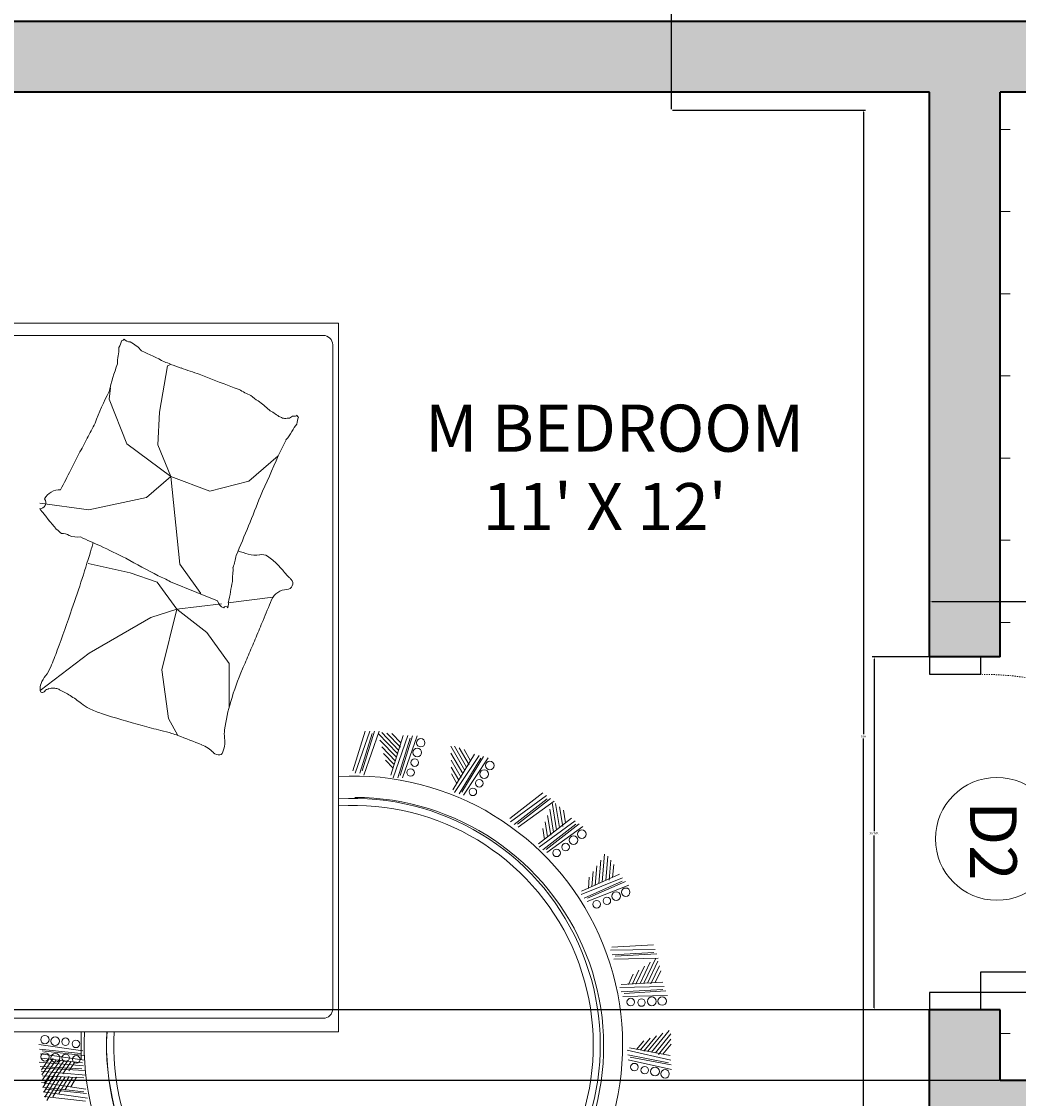
# Model space of a CAD drawing. Units: inches. Extents: x 2701 to 6846, y 811 to 2447.
# Tile 11 of 20: x 2841 to 2926, y 1371 to 1462. Entities that reach past the tile are written whole.
import ezdxf

# ---------------------------------------------------------------- set-up
doc = ezdxf.new("R2010")
doc.units = ezdxf.units.IN
doc.linetypes.add('HIDDEN4', pattern=[0.09375, 0.0625, -0.03125])
for name, color, linetype, lineweight in [('A-ANNO-DIMS', 2, 'Continuous', 18), ('A-ANNO-IDEN', 7, 'Continuous', 13), ('A-AREA-IDEN', 7, 'Continuous', 18), ('A-DOOR', 4, 'Continuous', 25), ('A-DOOR-SWNG', 4, 'HIDDEN4', 13), ('A-FLOR-PATT', 252, 'Continuous', 13), ('A-FURN', 8, 'Continuous', 13), ('A-WALL', 7, 'Continuous', 35)]:
    doc.layers.add(name, color=color, linetype=linetype, lineweight=lineweight)
doc.layers.add('A-WALL-PATT', color=18, linetype='Continuous', lineweight=13, true_color=0x000000)
doc.styles.add('DIM_FONT', font='SIMPLEX.shx', dxfattribs={"width": 0.8})
doc.styles.get("Standard").update_dxf_attribs({"font": 'arial.ttf'})
doc.dimstyles.get("Standard").update_dxf_attribs({"dimtxt": 0.18, "dimasz": 0.18, "dimexe": 0.18, "dimexo": 0.0625, "dimgap": 0.09, "dimtad": 0, "dimtih": 1, "dimtoh": 1, "dimdec": 4, "dimzin": 0, "dimdsep": 46, "dimtxsty": 'Standard', "dimcen": 0.09, "dimadec": 0, "dimazin": 0, "dimtfac": 1, "dimtdec": 4, "dimtofl": 0, "dimtmove": 0, "dimatfit": 3, "dimfxl": 1, "dimtolj": 1, "dimtzin": 0, "dimarcsym": 0})

# ---------------------------------------------------------------- blocks, each defined once
blk = doc.blocks.new('A$C187B6359')
for p, q in [((0.6999, 2.7053), (0.6999, 0.7053)), ((2.1999, 0.7053), (2.1999, 2.7053)), ((2.1741, 2.1968), (2.1741, 0.7375)), ((0.7284, 0.7375), (0.7284, 1.7894)), ((0.5629, 1.3285), (0.5533, 1.2408)), ((0.6047, 1.292), (0.5545, 1.3229)), ((0.5727, 1.3302), (0.5591, 1.2368)), ((0.6051, 1.3), (0.5613, 1.327)), ((0.5785, 1.3262), (0.5689, 1.2385)), ((0.6077, 1.3067), (0.5719, 1.3288)), ((0.5825, 1.332), (0.5729, 1.2443)), ((0.5923, 1.3337), (0.5787, 1.2403)), ((0.6059, 1.3161), (0.5826, 1.3304)), ((0.6394, 1.2947), (0.5911, 1.3283)), ((0.6403, 1.3027), (0.5981, 1.332)), ((0.6068, 1.3321), (0.6021, 1.244)), ((0.6165, 1.3344), (0.6081, 1.2403)), ((0.6432, 1.3092), (0.6087, 1.3332)), ((0.6225, 1.3307), (0.6178, 1.2426)), ((0.642, 1.3186), (0.6195, 1.3342)), ((0.6262, 1.3367), (0.6215, 1.2486)), ((0.6358, 1.339), (0.6275, 1.2449)), ((0.6437, 1.3345), (0.6342, 1.2469)), ((0.6535, 1.3363), (0.6399, 1.2428)), ((0.6593, 1.3323), (0.6497, 1.2446)), ((0.6633, 1.3381), (0.6538, 1.2504)), ((0.6731, 1.3398), (0.6595, 1.2463)), ((1.4224, 1.3369), (1.5015, 1.233)), ((1.8189, 1.3371), (1.8052, 1.2339)), ((0.6042, 1.284), (0.5618, 1.3102)), ((0.6385, 1.2867), (0.5976, 1.3152)), ((0.6387, 1.278), (0.6041, 1.3021)), ((0.6049, 1.2753), (0.569, 1.2975)), ((0.6034, 1.268), (0.5762, 1.2848)), ((0.6368, 1.2708), (0.6105, 1.289)), ((0.6035, 1.2597), (0.5834, 1.2721)), ((0.6364, 1.2624), (0.617, 1.2759)), ((0.6999, 1.25), (0.641, 1.25)), ((1.5015, 1.233), (1.5767, 1.1026)), ((1.6715, 1.1461), (1.6913, 1.235)), ((1.8052, 1.2339), (1.831, 1.1119)), ((1.9445, 1.1532), (2.0391, 1.191)), ((2.0391, 1.191), (2.0632, 1.1875)), ((1.6518, 1.0888), (1.6715, 1.1461)), ((1.8757, 1.0603), (1.9445, 1.1532)), ((1.5767, 1.1026), (1.5944, 1.0473)), ((1.831, 1.1119), (1.8757, 1.0603)), ((1.466, 1.0789), (1.3632, 1.0651)), ((1.5944, 1.0473), (1.466, 1.0789)), ((1.5944, 1.0473), (1.6518, 1.0888)), ((1.8757, 1.0603), (1.9428, 1.0878)), ((1.9428, 1.0878), (2.0116, 1.0844)), ((2.0116, 1.0844), (2.1096, 1.0672)), ((1.3632, 1.0651), (1.3272, 1.045)), ((1.6527, 1.0611), (1.6296, 1.0048)), ((1.8757, 1.0603), (1.6899, 1.0414)), ((1.8447, 0.9778), (1.8757, 1.0603)), ((2.1096, 1.0672), (2.1129, 1.0608)), ((1.545, 0.9841), (1.5944, 1.0473)), ((1.5944, 1.0473), (1.6062, 0.9532)), ((1.6899, 1.0414), (1.64, 1.0053)), ((1.6296, 1.0048), (1.6119, 0.9614)), ((1.64, 1.0053), (1.628, 0.9967)), ((1.4798, 0.9367), (1.545, 0.9841)), ((1.8654, 0.8953), (1.8447, 0.9778)), ((1.3869, 0.9367), (1.4798, 0.9367)), ((1.6081, 0.9385), (1.6199, 0.8439)), ((1.919, 0.8327), (1.8654, 0.8953)), ((2.1541, 0.7175), (0.7484, 0.7175)), ((0.6999, 0.7053), (2.1999, 0.7053)), ((1.3363, 0.639), (1.2472, 0.6702)), ((1.3365, 0.6489), (1.2523, 0.6751)), ((1.336, 0.619), (1.243, 0.6516)), ((1.3313, 0.6341), (1.2471, 0.6602)), ((1.3362, 0.629), (1.252, 0.6552)), ((1.281, 0.5827), (1.3169, 0.6174)), ((1.2887, 0.5803), (1.331, 0.6213)), ((1.327, 0.5684), (1.2428, 0.5946)), ((1.2576, 0.5894), (1.2746, 0.6058)), ((1.2657, 0.5875), (1.2887, 0.6097)), ((1.2725, 0.5842), (1.3028, 0.6136)), ((1.2964, 0.5779), (1.3333, 0.6137)), ((1.3022, 0.5738), (1.3324, 0.6031)), ((1.3218, 0.5536), (1.2375, 0.5798)), ((1.3268, 0.5585), (1.2377, 0.5897)), ((1.3267, 0.5485), (1.2424, 0.5747)), ((1.3117, 0.5732), (1.3313, 0.5922)), ((1.3265, 0.5386), (1.2374, 0.5698)), ((1.2849, 0.4076), (1.2061, 0.4596)), ((1.2875, 0.4172), (1.2122, 0.4631)), ((1.2253, 0.4544), (1.2458, 0.4663)), ((1.2327, 0.4506), (1.2604, 0.4666)), ((1.2385, 0.4458), (1.275, 0.4669)), ((1.2464, 0.4422), (1.2896, 0.4672)), ((1.2533, 0.4381), (1.3042, 0.4675)), ((1.2601, 0.4339), (1.3046, 0.4596)), ((1.2798, 0.3883), (1.2009, 0.4403)), ((1.2788, 0.4041), (1.2035, 0.45)), ((1.2824, 0.398), (1.207, 0.4439)), ((1.2647, 0.4284), (1.3012, 0.4495)), ((1.2738, 0.4255), (1.2975, 0.4392)), ((1.2056, 0.2727), (1.1513, 0.3422)), ((1.1882, 0.2484), (1.1328, 0.3249)), ((1.1929, 0.2635), (1.1386, 0.333)), ((1.194, 0.2565), (1.1397, 0.3261)), ((1.1998, 0.2646), (1.1444, 0.3411)), ((1.1461, 0.2039), (1.0907, 0.2804)), ((1.1519, 0.212), (1.0976, 0.2815)), ((1.1345, 0.1877), (1.0791, 0.2642)), ((1.1392, 0.2028), (1.0849, 0.2723)), ((1.1403, 0.1958), (1.086, 0.2653)), ((1.1069, 0.2688), (1.1302, 0.2726)), ((1.1124, 0.2626), (1.144, 0.2678)), ((1.1161, 0.256), (1.1577, 0.2629)), ((1.1223, 0.2499), (1.1715, 0.2581)), ((1.1272, 0.2436), (1.1853, 0.2532)), ((1.1322, 0.2373), (1.1829, 0.2457)), ((1.1346, 0.2306), (1.1761, 0.2374)), ((1.142, 0.2247), (1.169, 0.2291)), ((1.0187, 0.1044), (0.9829, 0.185)), ((1.0257, 0.1038), (0.9905, 0.1915)), ((1.0333, 0.1102), (0.9976, 0.1909)), ((1.0105, 0.0909), (0.9754, 0.1786)), ((1.0181, 0.0974), (0.9824, 0.178)), ((1.0034, 0.1763), (1.027, 0.1743)), ((1.0073, 0.1689), (1.0391, 0.1663)), ((1.0093, 0.1617), (1.0513, 0.1582)), ((1.0138, 0.1542), (1.0635, 0.1501)), ((1.017, 0.1469), (1.0757, 0.1421)), ((1.0203, 0.1396), (1.0715, 0.1353)), ((0.8555, 0.0282), (0.8535, 0.1226)), ((0.8649, 0.0315), (0.8599, 0.1196)), ((0.8679, 0.0379), (0.8629, 0.1259)), ((0.8743, 0.0349), (0.8723, 0.1293)), ((0.8837, 0.0382), (0.8787, 0.1263)), ((1.021, 0.1325), (1.0629, 0.129)), ((1.0268, 0.1249), (1.0541, 0.1227)), ((0.6197, 0), (0.6408, 0.0921)), ((0.6341, 0.0064), (0.6507, 0.093)), ((0.6396, 0.0019), (0.6606, 0.094)), ((0.7768, 0.0089), (0.7748, 0.1033)), ((0.7862, 0.0122), (0.7812, 0.1003)), ((0.7892, 0.0186), (0.7842, 0.1066)), ((0.7956, 0.0156), (0.7936, 0.11)), ((0.805, 0.0189), (0.7999, 0.107)), ((0.8003, 0.0912), (0.8216, 0.0811)), ((0.6296, 0.001), (0.6463, 0.0876)), ((0.6495, 0.0029), (0.6661, 0.0895)), ((0.6626, 0.0742), (0.6808, 0.0592)), ((0.8006, 0.0755), (0.8387, 0.0574)), ((0.8013, 0.083), (0.8302, 0.0693)), ((0.6585, 0.0501), (0.697, 0.0184)), ((0.659, 0.0588), (0.6916, 0.032)), ((0.6615, 0.0659), (0.6862, 0.0456)), ((0.8022, 0.0669), (0.8473, 0.0456)), ((0.8027, 0.0589), (0.8559, 0.0337)), ((0.8031, 0.0509), (0.8496, 0.0289)), ((0.652, 0.0281), (0.6845, 0.0014)), ((0.6555, 0.0344), (0.6952, 0.0017)), ((0.657, 0.0423), (0.7025, 0.0049)), ((0.8013, 0.044), (0.8393, 0.026)), ((0.804, 0.0349), (0.8288, 0.0232)), ((0.6525, 0.0186), (0.6736, 0.0013))]:
    blk.add_line(p, q)
for centre, radius in [((0.6466, 1.3265), 0.00895), ((0.6832, 1.3267), 0.00895), ((0.6447, 1.3047), 0.00929), ((0.68, 1.3051), 0.00929), ((0.6447, 1.2827), 0.00801), ((0.6788, 1.2831), 0.00801), ((0.6414, 1.2602), 0.00801), ((0.6743, 1.2609), 0.00801), ((1.2488, 0.5526), 0.00801), ((1.2698, 0.5438), 0.00801), ((1.2911, 0.5385), 0.00929), ((1.3118, 0.5312), 0.00895), ((1.2078, 0.4208), 0.00801), ((1.226, 0.4072), 0.00801), ((1.2454, 0.3969), 0.00929), ((1.2637, 0.3848), 0.00895), ((1.0786, 0.2435), 0.00801), ((1.0909, 0.2244), 0.00801), ((1.1054, 0.2078), 0.00929), ((1.1182, 0.1901), 0.00895), ((0.9699, 0.1587), 0.00801), ((0.9771, 0.1371), 0.00801), ((0.9871, 0.1175), 0.00929), ((0.7627, 0.0865), 0.00801), ((0.9953, 0.0972), 0.00895), ((0.625, 0.0788), 0.00801), ((0.7618, 0.0638), 0.00801), ((0.6186, 0.057), 0.00801), ((0.7643, 0.042), 0.00929), ((0.6108, 0.0139), 0.00895), ((0.6157, 0.0352), 0.00929), ((0.7648, 0.0201), 0.00895)]:
    blk.add_circle(centre, radius)
for centre, radius, start, end in [((1.4245, 1.3321), 0.0063, 166.7192, 233.4208), ((1.4227, 1.3325), 0.00443, 93.9484, 166.7192), ((1.4123, 1.3157), 0.0142, 10.4074, 53.4208), ((1.4248, 1.3018), 0.0352, 69.6548, 93.9484), ((1.4161, 1.2784), 0.0601, 51.4146, 69.6548), ((1.503, 1.3874), 0.0792, 231.4146, 247.2931), ((1.3919, 1.8509), 0.6605, 306.2163, 307.2151), ((2.0244, 1.0216), 0.3825, 126.2163, 127.5287), ((1.8298, 1.2978), 0.0452, 127.5287, 134.1274), ((1.7586, 1.3879), 0.0697, 308.8136, 314.1274), ((1.8199, 1.3372), 0.0127, 176.7545, 308.8136), ((1.8114, 1.2954), 0.0359, 356.7545, 62.7098), ((1.3889, 1.3133), 0.0393, 333.1821, 345.4291), ((1.3504, 1.3043), 0.0771, 2.7286, 10.4074), ((1.4121, 1.3072), 0.0153, 345.4291, 2.7286), ((1.7956, 2.0865), 0.8371, 247.2931, 249.8713), ((3.2606, 6.0836), 5.0942, 249.8713, 250.9164), ((1.7012, 1.3479), 0.0774, 313.5224, 324.1064), ((1.6323, 1.4759), 0.2176, 307.2151, 313.5224), ((1.1098, 1.4543), 0.352, 329.0944, 333.1821), ((1.7321, 1.2886), 0.0226, 324.1064, 8.0492), ((0.4694, -1.4805), 3.0972, 62.7098, 63.5853), ((1.2454, 1.3732), 0.194, 320.2995, 329.0944), ((2.6233, 4.2415), 3.145, 250.9164, 253.3915), ((1.7928, 1.2579), 0.0458, 157.5838, 188.0492), ((2.8204, 3.0604), 2.0162, 242.5001, 243.5853), ((4.7738, 6.6498), 6.1019, 242.15178, 242.50014), ((0.6715, 0.6736), 0.5699, 87.1307, 3.1127), ((1.5607, 1.1468), 0.1965, 153.9265, 162.1604), ((1.457, 1.1975), 0.081, 140.2995, 153.9265), ((2.6582, 0.8258), 1.0054, 154.9471, 157.5838), ((-0.7388, -3.9416), 5.8383, 62.15178, 62.50792), ((3.2306, 0.441), 1.6868, 152.9116, 154.9471), ((1.7577, 1.3394), 0.1166, 253.3915, 259.2634), ((1.7675, 0.6374), 0.6236, 62.5079, 69.2514), ((0.6698, 0.67), 0.5261, 86.7143, 0.065), ((0.6715, 0.6736), 0.5225, 86.8806, 3.3918), ((3.2804, 0.5933), 2.003, 162.1604, 164.7375), ((1.9614, 0.771), 0.43, 69.2514, 77.3748), ((0.6715, 0.6735), 0.5076, 86.694, 3.4914), ((2.1175, 1.1102), 0.063, 77.3748, 93.3881), ((2.1447, 1.23), 0.0599, 256.9598, 273.3881), ((2.175, 1.2135), 0.0509, 238.3083, 256.9598), ((2.1693, 1.1641), 0.0058, 180.9614, 238.3083), ((3.0589, 0.3742), 1.5652, 150.064, 152.9116), ((2.0927, 1.1796), 0.0755, 310.5086, 333.6668), ((2.1772, 1.1464), 0.0168, 130.5086, 180.9614), ((2.938, 0.6868), 1.6481, 164.7375, 166.159), ((-0.2673, 2.2544), 2.6619, 333.6668, 334.8268), ((0.8082, 1.2115), 0.5454, 343.6878, 346.159), ((1.4669, 1.1681), 0.2143, 330.064, 337.7645), ((1.9502, 1.1372), 0.1798, 334.8268, 339.2919), ((1.1591, 1.1088), 0.1798, 339.2227, 343.6878), ((1.5949, 1.2314), 0.5454, 339.2919, 341.7631), ((-1.1616, 1.9893), 2.6619, 338.0627, 339.2227), ((3.6572, 0.4841), 1.6481, 160.3416, 161.7631), ((1.2375, 1.0231), 0.0755, 314.9045, 338.0627), ((3.9459, 0.2419), 2.003, 157.7645, 160.3416), ((1.3026, 0.9577), 0.0168, 134.9045, 185.3572), ((1.6187, 0.9393), 0.0231, 107.1867, 157.7645), ((1.2917, 0.9567), 0.0058, 185.3572, 242.7041), ((1.3124, 0.9968), 0.0509, 242.7041, 261.3557), ((1.3137, 1.0056), 0.0599, 261.3557, 277.784), ((1.3304, 0.8839), 0.063, 81.7707, 97.784), ((1.2779, 0.5207), 0.43, 73.6473, 81.7707), ((1.5958, 0.9437), 0.00467, 287.1867, 70.6201), ((1.5979, 0.93), 0.0092, 70.6201, 94.2593), ((1.6056, 0.9723), 0.034, 262.0178, 274.2593), ((1.6584, 1.1274), 0.1955, 255.1193, 262.0178), ((1.2233, 0.3349), 0.6236, 66.9038, 73.6473), ((1.6072, 0.7561), 0.1794, 75.1193, 82.3216), ((1.6589, 0.8584), 0.0712, 82.3216, 94.5118), ((1.6778, 0.9947), 0.0663, 261.8784, 274.5118), ((1.7248, 1.0373), 0.1166, 248.9957, 261.8784), ((2.9614, 3.8066), 3.145, 246.5205, 248.9957), ((2.6668, 0.5851), 1.0054, 160.6552, 161.9797), ((2.229, 0.8161), 0.1965, 149.5306, 157.7645), ((-0.8223, -4.4619), 5.8383, 66.54766, 66.9038), ((3.9298, 6.492), 6.1019, 246.54766, 246.89602), ((1.7543, 0.882), 0.0458, 161.9797, 192.4451), ((2.1053, 0.8341), 0.081, 135.9036, 149.5306), ((2.3266, 2.7341), 2.0162, 246.896, 247.9812), ((1.6874, 0.8672), 0.0226, 328.5023, 12.4451), ((3.9486, 5.5052), 5.0942, 245.4754, 246.5205), ((1.8771, 0.9873), 0.194, 315.9036, 324.6985), ((0.4095, -2.0064), 3.0972, 67.1056, 67.9812), ((1.6004, 0.8138), 0.0359, 1.1504, 67.1056), ((1.5366, 0.9898), 0.2176, 311.611, 317.9183), ((1.6407, 0.8959), 0.0774, 317.9183, 328.5023), ((1.7154, 1.0347), 0.352, 324.6985, 328.7862), ((1.2426, 1.321), 0.6605, 310.6122, 311.611), ((2.3003, 1.5779), 0.8371, 242.8972, 245.4754), ((1.9838, 0.8242), 0.0153, 341.0332, 358.3327), ((1.9655, 0.8441), 0.0393, 328.7862, 341.0332), ((1.649, 0.8147), 0.0127, 181.1504, 313.2095), ((1.61, 0.8562), 0.0697, 313.2095, 318.5233), ((1.6961, 0.7801), 0.0452, 131.9246, 138.5233), ((1.9215, 0.5292), 0.3825, 130.6122, 131.9246), ((2.0069, 0.8743), 0.0792, 227.0187, 242.8972), ((1.9456, 0.7491), 0.0601, 47.0187, 65.2589), ((1.9216, 0.8111), 0.0771, 358.3327, 6.0115), ((1.9894, 0.7982), 0.0142, 6.0115, 49.0249), ((2.0095, 0.7978), 0.0063, 162.3233, 229.0249), ((1.9863, 0.7579), 0.0352, 65.2589, 89.5525), ((2.0053, 0.7886), 0.00443, 89.5525, 162.3233), ((0.7484, 0.7375), 0.02, 180, 270), ((2.1541, 0.7375), 0.02, 270, 0)]:
    blk.add_arc(centre, radius, start, end)
at = {"style": 'DIM_FONT', "text_generation_flag": 4, "width": 0.8, "flags": 9}
for tag in ['YSIZE', 'XSIZE']:
    blk.add_attdef(tag, (2.1999, 2.7053), '', height=0.0005, rotation=180, dxfattribs=at)
blk = doc.blocks.new('DOOR-D2-30IN-PANEL-FRAME')
blk.add_lwpolyline([(0, 30), (0, 28.521), (4.361, 28.521), (4.361, 30), (0, 30)], close=True)
for points in [[(3.925, 30), (0.436, 30)], [(4.361, 0), (4.361, 3.224), (31.403, 3.224), (31.403, 1.479), (0, 1.479), (0, 0)], [(0, 0), (4.361, 0)], [(3.925, 0), (0.436, 0)]]:
    blk.add_lwpolyline(points)
blk = doc.blocks.new('*D29')
at = {"layer": 'A-ANNO-DIMS', "color": 0, "lineweight": -2, "transparency": 16777216}
for p, q in [((2917.971, 1408.113), (2917.971, 1412.94)), ((2918.151, 1412.76), (2932.954, 1412.76)), ((2949.194, 1412.76), (2934.392, 1412.76)), ((2949.374, 1408.113), (2949.374, 1412.94))]:
    blk.add_line(p, q, dxfattribs=at)
at = {"layer": 'A-ANNO-DIMS', "color": 0, "transparency": 16777216}
for points in [[(2918.151, 1412.79), (2918.151, 1412.73), (2917.971, 1412.76)], [(2949.194, 1412.79), (2949.194, 1412.73), (2949.374, 1412.76)]]:
    blk.add_solid(points, dxfattribs=at)
at = {"layer": 'Defpoints', "color": 0, "transparency": 16777216}
for p in [(2949.374, 1412.76), (2917.971, 1408.05), (2949.374, 1408.05)]:
    blk.add_point(p, dxfattribs=at)
at = {"layer": 'A-ANNO-DIMS', "color": 0, "transparency": 16777216, "insert": (2933.673, 1412.76), "char_height": 0.18, "attachment_point": 5}
blk.add_mtext('\\A1;D2 31 TYP.', dxfattribs=at)
blk = doc.blocks.new('*D30')
at = {"layer": 'A-ANNO-DIMS', "color": 0, "lineweight": -2, "transparency": 16777216}
for p, q in [((2917.909, 1408.05), (2913.081, 1408.05)), ((2913.261, 1407.87), (2913.261, 1393.232)), ((2913.261, 1378.23), (2913.261, 1392.868)), ((2917.909, 1378.05), (2913.081, 1378.05))]:
    blk.add_line(p, q, dxfattribs=at)
at = {"layer": 'A-ANNO-DIMS', "color": 0, "transparency": 16777216}
for points in [[(2913.231, 1407.87), (2913.291, 1407.87), (2913.261, 1408.05)], [(2913.231, 1378.23), (2913.291, 1378.23), (2913.261, 1378.05)]]:
    blk.add_solid(points, dxfattribs=at)
at = {"layer": 'Defpoints', "color": 0, "transparency": 16777216}
for p in [(2913.261, 1408.05), (2917.971, 1408.05), (2917.971, 1378.05)]:
    blk.add_point(p, dxfattribs=at)
at = {"layer": 'A-ANNO-DIMS', "color": 0, "transparency": 16777216, "insert": (2913.261, 1393.05), "char_height": 0.18, "attachment_point": 5}
blk.add_mtext('\\A1;30 TYP.', dxfattribs=at)
blk = doc.blocks.new('*D49')
at = {"layer": 'A-ANNO-DIMS', "color": 0, "lineweight": -2, "transparency": 16777216}
for p, q in [((2787.416, 1454.59), (2787.416, 1471.002)), ((2896.043, 1454.59), (2896.043, 1471.002)), ((2787.596, 1470.822), (2840.655, 1470.822)), ((2895.863, 1470.822), (2842.804, 1470.822))]:
    blk.add_line(p, q, dxfattribs=at)
at = {"layer": 'A-ANNO-DIMS', "color": 0, "transparency": 16777216}
for points in [[(2787.596, 1470.852), (2787.596, 1470.792), (2787.416, 1470.822)], [(2895.863, 1470.852), (2895.863, 1470.792), (2896.043, 1470.822)]]:
    blk.add_solid(points, dxfattribs=at)
at = {"layer": 'Defpoints', "color": 0, "transparency": 16777216}
for p in [(2787.416, 1470.822), (2787.416, 1454.528), (2896.043, 1454.528)]:
    blk.add_point(p, dxfattribs=at)
at = {"layer": 'A-ANNO-DIMS', "color": 0, "transparency": 16777216, "insert": (2841.729, 1470.822), "char_height": 0.18, "attachment_point": 5}
blk.add_mtext('\\A1;BED GROUP 109', dxfattribs=at)
blk = doc.blocks.new('*D50')
at = {"layer": 'A-ANNO-DIMS', "color": 0, "lineweight": -2, "transparency": 16777216}
for p, q in [((2896.105, 1454.528), (2912.517, 1454.528)), ((2912.337, 1454.348), (2912.337, 1401.492)), ((2912.337, 1348.272), (2912.337, 1401.128)), ((2896.105, 1348.092), (2912.517, 1348.092))]:
    blk.add_line(p, q, dxfattribs=at)
at = {"layer": 'A-ANNO-DIMS', "color": 0, "transparency": 16777216}
for points in [[(2912.307, 1454.348), (2912.367, 1454.348), (2912.337, 1454.528)], [(2912.307, 1348.272), (2912.367, 1348.272), (2912.337, 1348.092)]]:
    blk.add_solid(points, dxfattribs=at)
at = {"layer": 'Defpoints', "color": 0, "transparency": 16777216}
for p in [(2896.043, 1454.528), (2912.337, 1454.528), (2896.043, 1348.092)]:
    blk.add_point(p, dxfattribs=at)
at = {"layer": 'A-ANNO-DIMS', "color": 0, "transparency": 16777216, "insert": (2912.337, 1401.31), "char_height": 0.18, "attachment_point": 5}
blk.add_mtext('\\A1;106', dxfattribs=at)
blk = doc.blocks.new('*D75')
at = {"layer": 'A-ANNO-DIMS', "color": 0, "lineweight": -2, "transparency": 16777216}
for p, q in [((2923.909, 1378.05), (2700.591, 1378.05)), ((2700.771, 1377.87), (2700.771, 1375.232)), ((2700.771, 1372.23), (2700.771, 1374.868)), ((2923.909, 1372.05), (2700.591, 1372.05))]:
    blk.add_line(p, q, dxfattribs=at)
at = {"layer": 'A-ANNO-DIMS', "color": 0, "transparency": 16777216}
for points in [[(2700.741, 1377.87), (2700.801, 1377.87), (2700.771, 1378.05)], [(2700.741, 1372.23), (2700.801, 1372.23), (2700.771, 1372.05)]]:
    blk.add_solid(points, dxfattribs=at)
at = {"layer": 'Defpoints', "color": 0, "transparency": 16777216}
for p in [(2700.771, 1378.05), (2923.971, 1378.05), (2923.971, 1372.05)]:
    blk.add_point(p, dxfattribs=at)
at = {"layer": 'A-ANNO-DIMS', "color": 0, "transparency": 16777216, "insert": (2700.771, 1375.05), "char_height": 0.18, "attachment_point": 5}
blk.add_mtext('\\A1;6', dxfattribs=at)

msp = doc.modelspace()

# ---------------------------------------------------------------- hatches: boundary and pattern name
at = {"layer": 'A-FLOR-PATT'}
h = msp.add_hatch(dxfattribs=at)
h.set_pattern_fill('ANGLE', color=256)
h.set_pattern_definition([(0, (0, 0), (0, 6.985), [5.08, -1.905]), (90, (0, 0), (-6.985, 4e-16), [5.08, -1.905])])
h.paths.add_polyline_path([(2841.813, 1296.511, -0.109453), (2842.614, 1300.129, -0.102375), (2844.977, 1303.302, -0.093743), (2848.426, 1305.368, -0.062463), (2851.367, 1306.05), (2785.971, 1306.05), (2785.971, 1258.05), (2827.971, 1258.05), (2827.971, 1256.412), (2829.451, 1256.412, -0.394827), (2854.747, 1283.453), (2856.492, 1283.453), (2856.492, 1256.412), (2857.971, 1256.412), (2857.971, 1258.05), (2863.971, 1258.05), (2863.971, 1306.05), (2853.867, 1306.05, -0.062463), (2856.808, 1305.368, -0.093743), (2860.257, 1303.302, -0.102375), (2862.62, 1300.129, -0.109453), (2863.421, 1296.511, -0.109453), (2862.62, 1292.893, -0.102375), (2860.257, 1289.72, -0.093738), (2856.808, 1287.654, -0.088425), (2852.617, 1286.907, -0.088425), (2848.426, 1287.654, -0.093738), (2844.977, 1289.72, -0.102375), (2842.614, 1292.893, -0.109453)])
h.paths.add_polyline_path([(2805.215, 1273.877, -0.141745), (2808.319, 1271.773, -0.184983), (2809.774, 1267.974, -0.184983), (2808.319, 1264.176, -0.141745), (2805.215, 1262.071, -0.152244), (2799.994, 1261.796, -0.025614), (2799.369, 1261.945), (2794.365, 1263.418), (2794.365, 1263.405, -0.111242), (2793.993, 1261.915, -0.033889), (2793.114, 1260.114, -0.286745), (2792.376, 1259.652), (2787.581, 1259.652, -0.414214), (2787.153, 1260.08), (2787.153, 1267.974), (2787.153, 1275.869, -0.414214), (2787.581, 1276.297), (2792.376, 1276.297, -0.286745), (2793.114, 1275.835, -0.033889), (2793.993, 1274.033, -0.105104), (2794.362, 1272.628), (2794.365, 1272.53), (2799.369, 1274.003, -0.025614), (2799.994, 1274.153, -0.152244)], flags=16)
h.paths.add_polyline_path([(2804.681, 1272.34, -0.144945), (2807.088, 1270.709, -0.0358), (2807.447, 1270.253, -0.133285), (2807.893, 1268.608), (2807.893, 1267.974), (2807.893, 1267.341, -0.133285), (2807.447, 1265.696, -0.0358), (2807.088, 1265.24, -0.144945), (2804.681, 1263.609, -0.155404), (2800.343, 1263.386, -0.364511), (2796.485, 1267.974, -0.364511), (2800.343, 1272.563, -0.155404)], flags=0)
h.paths.add_polyline_path([(2800.016, 1268.901, 0.169298), (2799.131, 1268.116, 0.076667), (2799.1, 1267.974, 0.076667), (2799.131, 1267.833, 0.169298), (2800.016, 1267.047, 0.305219), (2800.365, 1267.156, 0.169535), (2800.651, 1267.974, 0.169535), (2800.365, 1268.792, 0.305219)], flags=0)
h.paths.add_polyline_path([(2971.971, 1456.05), (2923.971, 1456.05), (2923.971, 1408.05), (2922.333, 1408.05), (2922.333, 1406.571, -0.394827), (2949.374, 1381.274), (2949.374, 1379.529), (2922.333, 1379.529), (2922.333, 1378.05), (2923.971, 1378.05), (2923.971, 1372.05), (2971.971, 1372.05)])
h.paths.add_polyline_path([(2939.818, 1436.526, -0.141745), (2937.713, 1433.423, -0.184983), (2933.915, 1431.968, -0.184983), (2930.117, 1433.423, -0.141745), (2928.012, 1436.526, -0.152244), (2927.736, 1441.747, -0.025614), (2927.886, 1442.373), (2929.359, 1447.376), (2929.346, 1447.377, -0.111242), (2927.856, 1447.748, -0.033889), (2926.054, 1448.627, -0.286745), (2925.593, 1449.366), (2925.593, 1454.16, -0.414214), (2926.021, 1454.589), (2933.915, 1454.589), (2941.809, 1454.589, -0.414207), (2942.237, 1454.16), (2942.237, 1449.366, -0.286745), (2941.776, 1448.627, -0.033889), (2939.974, 1447.748, -0.105104), (2938.569, 1447.38), (2938.471, 1447.376), (2939.944, 1442.373, -0.025614), (2940.094, 1441.747, -0.152244)], flags=16)
h.paths.add_polyline_path([(2938.281, 1437.06, -0.144945), (2936.649, 1434.654, -0.0358), (2936.193, 1434.294, -0.133285), (2934.548, 1433.848), (2933.915, 1433.848), (2933.281, 1433.848, -0.133285), (2931.636, 1434.294, -0.0358), (2931.181, 1434.654, -0.144945), (2929.549, 1437.06, -0.155404), (2929.326, 1441.398, -0.364511), (2933.915, 1445.256, -0.364511), (2938.503, 1441.398, -0.155404)], flags=0)
h.paths.add_polyline_path([(2969.158, 1392.045, -0.093743), (2971.224, 1388.596, -0.088421), (2971.971, 1384.405, -0.088421), (2971.224, 1380.214, -0.093743), (2969.158, 1376.765, -0.102375), (2965.986, 1374.402, -0.109453), (2962.367, 1373.6, -0.109453), (2958.749, 1374.402, -0.102375), (2955.576, 1376.765, -0.093738), (2953.511, 1380.213, -0.088425), (2952.764, 1384.405, -0.088425), (2953.511, 1388.596, -0.093738), (2955.576, 1392.045, -0.102375), (2958.749, 1394.407, -0.109453), (2962.367, 1395.209, -0.109453), (2965.986, 1394.407, -0.102375)], flags=0)
edge = h.paths.add_edge_path(flags=16)
edge.add_arc((2961.075, 1384.859), 10.199, 20.2132, 41.63359, ccw=False)
edge.add_spline(control_points=[(2970.646, 1388.383), (2970.459, 1387.83), (2970.004, 1386.481), (2971.435, 1384.396), (2969.868, 1382.339), (2970.408, 1381.011), (2970.646, 1380.426)], knot_values=[0, 0, 0, 0, 0.041109, 0.100337, 0.155913, 0.199586, 0.199586, 0.199586, 0.199586], degree=3, periodic=0)
edge.add_arc((2961.075, 1383.95), 10.199, 318.36641, 339.7868, ccw=False)
edge.add_arc((2961.862, 1383.25), 9.145, 294.98529, 318.36641, ccw=False)
edge.add_arc((2962.367, 1382.166), 7.949, 269.99999, 294.98535, ccw=False)
edge.add_arc((2962.367, 1382.166), 7.949, 245.01465, 270.00002, ccw=False)
edge.add_arc((2962.873, 1383.25), 9.145, 221.63359, 245.01471, ccw=False)
edge.add_arc((2963.66, 1383.95), 10.199, 200.21296, 221.63359, ccw=False)
edge.add_arc((2964.894, 1384.405), 11.514, 180, 200.21296, ccw=False)
edge.add_arc((2964.894, 1384.405), 11.514, 159.78704, 179.99999, ccw=False)
edge.add_arc((2963.66, 1384.859), 10.199, 138.36641, 159.78704, ccw=False)
edge.add_arc((2962.873, 1385.559), 9.145, 114.98529, 138.36641, ccw=False)
edge.add_arc((2962.367, 1386.643), 7.949, 89.99999, 114.98534, ccw=False)
edge.add_arc((2962.367, 1386.643), 7.949, 65.01465, 90.00002, ccw=False)
edge.add_arc((2961.862, 1385.559), 9.145, 41.63359, 65.01471, ccw=False)
h.paths.add_polyline_path([(2963.81, 1393.327, -0.126458), (2966.613, 1390.683, -0.141697), (2967.169, 1388.761), (2967.169, 1387.406, -1), (2969.57, 1387.406, -0.414214), (2968.37, 1386.205), (2963.568, 1385.005, 0.146218), (2963.311, 1384.663), (2968.97, 1385.64), (2968.97, 1383.155), (2963.317, 1384.13, 0.140312), (2963.568, 1383.804), (2968.37, 1382.604, -0.414214), (2969.57, 1381.403, -1), (2967.169, 1381.403), (2967.169, 1380.04, -0.149025), (2966.557, 1378.032, -0.012759), (2966.265, 1377.619, -0.106303), (2963.81, 1375.482, -0.126822), (2961.167, 1374.801, -0.126822), (2958.524, 1375.482, -0.106303), (2956.069, 1377.619, -0.085722), (2954.537, 1380.623, -0.075351), (2953.964, 1384.405, -0.075351), (2954.537, 1388.187, -0.085722), (2956.069, 1391.19, -0.106303), (2958.524, 1393.327, -0.126822), (2961.167, 1394.009, -0.126822)], flags=0)
h.paths.add_polyline_path([(2934.842, 1441.725, 0.169298), (2934.056, 1442.61, 0.076667), (2933.915, 1442.641, 0.076667), (2933.773, 1442.61, 0.169298), (2932.988, 1441.725, 0.305219), (2933.097, 1441.376, 0.169535), (2933.915, 1441.09, 0.169535), (2934.733, 1441.376, 0.305219)], flags=0)
h.paths.add_polyline_path([(2969.324, 1387.406, -1), (2967.416, 1387.406, -1)], flags=0)
h.paths.add_polyline_path([(2968.831, 1387.406, -1), (2967.909, 1387.406, -1)], flags=0)
h.paths.add_polyline_path([(2962.13, 1384.357, -1), (2960.209, 1384.357, -1)], flags=0)
h.paths.add_polyline_path([(2961.801, 1384.357, -1), (2960.538, 1384.357, -1)], flags=0)
h.paths.add_polyline_path([(2969.324, 1381.403, -1), (2967.416, 1381.403, -1)], flags=0)
h.paths.add_polyline_path([(2968.831, 1381.403, -1), (2967.909, 1381.403, -1)], flags=0)
h.paths.add_polyline_path([(3085.971, 1306.05), (3001.971, 1306.05), (3001.971, 1300.05), (3000.333, 1300.05), (3000.333, 1298.571), (3027.374, 1298.571), (3027.374, 1296.826, -0.394827), (3000.333, 1271.529), (3000.333, 1270.05), (3001.971, 1270.05), (3001.971, 1258.05), (3085.971, 1258.05)])
h.paths.add_polyline_path([(3033.333, 1274.445, -0.102375), (3035.696, 1271.272, -0.109453), (3036.497, 1267.654, -0.109453), (3035.696, 1264.036, -0.102375), (3033.333, 1260.863, -0.093743), (3029.884, 1258.797, -0.088421), (3025.693, 1258.05, -0.088421), (3021.502, 1258.797, -0.093743), (3018.053, 1260.863, -0.102375), (3015.69, 1264.036, -0.109453), (3014.888, 1267.654, -0.109453), (3015.69, 1271.272, -0.102375), (3018.053, 1274.445, -0.093738), (3021.502, 1276.511, -0.088425), (3025.693, 1277.258, -0.088425), (3029.884, 1276.511, -0.093738)], flags=0)
edge = h.paths.add_edge_path(flags=16)
edge.add_arc((3026.847, 1267.149), 9.145, 24.98529, 48.36641, ccw=False)
edge.add_arc((3027.931, 1267.654), 7.949, -0.00001, 24.98534, ccw=False)
edge.add_arc((3027.931, 1267.654), 7.949, -24.98534, 0.00002, ccw=False)
edge.add_arc((3026.847, 1268.159), 9.145, 311.63359, 335.01471, ccw=False)
edge.add_arc((3026.147, 1268.947), 10.199, 290.2132, 311.63359, ccw=False)
edge.add_spline(control_points=[(3029.671, 1259.376), (3029.087, 1259.613), (3027.759, 1260.153), (3025.702, 1258.586), (3023.617, 1260.017), (3022.267, 1259.562), (3021.715, 1259.376)], knot_values=[0, 0, 0, 0, 0.043673, 0.099248, 0.158477, 0.199586, 0.199586, 0.199586, 0.199586], degree=3, periodic=0)
edge.add_arc((3025.239, 1268.947), 10.199, 228.36641, 249.7868, ccw=False)
edge.add_arc((3024.538, 1268.159), 9.145, 204.98529, 228.36641, ccw=False)
edge.add_arc((3023.454, 1267.654), 7.949, 179.99999, 204.98534, ccw=False)
edge.add_arc((3023.454, 1267.654), 7.949, 155.01465, 180.00002, ccw=False)
edge.add_arc((3024.538, 1267.149), 9.145, 131.63359, 155.01471, ccw=False)
edge.add_arc((3025.239, 1266.361), 10.199, 110.21296, 131.63359, ccw=False)
edge.add_arc((3025.693, 1265.127), 11.514, 90, 110.21296, ccw=False)
edge.add_arc((3025.693, 1265.127), 11.514, 69.78704, 89.99999, ccw=False)
edge.add_arc((3026.147, 1266.361), 10.199, 48.36641, 69.78704, ccw=False)
h.paths.add_polyline_path([(3032.478, 1273.952, -0.106303), (3034.615, 1271.497, -0.126822), (3035.297, 1268.854, -0.126822), (3034.615, 1266.212, -0.106303), (3032.478, 1263.757, -0.012759), (3032.066, 1263.464, -0.149025), (3030.057, 1262.852), (3028.694, 1262.852, -0.414214), (3029.895, 1261.652, -1), (3027.494, 1261.652), (3026.293, 1266.453, 0.140312), (3025.968, 1266.704), (3026.943, 1261.051), (3024.458, 1261.051), (3025.434, 1266.71, 0.146218), (3025.093, 1266.453), (3023.892, 1261.652, -1), (3021.491, 1261.652, -0.414214), (3022.692, 1262.852), (3021.337, 1262.852, -0.141697), (3019.415, 1263.408, -0.126458), (3016.77, 1266.212, -0.126822), (3016.089, 1268.854, -0.126822), (3016.77, 1271.497, -0.106303), (3018.908, 1273.952, -0.085722), (3021.911, 1275.484, -0.075351), (3025.693, 1276.057, -0.075351), (3029.475, 1275.484, -0.085722)], flags=0)
h.paths.add_polyline_path([(3072.365, 1280.002, -0.184983), (3076.163, 1281.457, -0.184983), (3079.961, 1280.002, -0.141745), (3082.066, 1276.898, -0.152244), (3082.342, 1271.678, -0.025614), (3082.192, 1271.052), (3080.719, 1266.048), (3080.817, 1266.045, -0.105104), (3082.222, 1265.676, -0.033889), (3084.024, 1264.798, -0.286745), (3084.485, 1264.059), (3084.485, 1259.264, -0.41422), (3084.057, 1258.836), (3076.163, 1258.836), (3068.269, 1258.836, -0.414214), (3067.841, 1259.264), (3067.841, 1264.059, -0.286745), (3068.302, 1264.798, -0.033889), (3070.104, 1265.676, -0.105104), (3071.509, 1266.045), (3071.607, 1266.048), (3070.134, 1271.052, -0.025614), (3069.984, 1271.678, -0.152244), (3070.26, 1276.898, -0.141745)], flags=16)
h.paths.add_polyline_path([(3073.429, 1278.771, -0.0358), (3073.885, 1279.13, -0.133285), (3075.529, 1279.577), (3076.163, 1279.577), (3076.797, 1279.577, -0.133285), (3078.441, 1279.13, -0.0358), (3078.897, 1278.771, -0.144945), (3080.529, 1276.364, -0.155404), (3080.752, 1272.026, -0.364511), (3076.163, 1268.168, -0.364511), (3071.574, 1272.026, -0.155404), (3071.797, 1276.364, -0.144945)], flags=0)
h.paths.add_polyline_path([(3026.7, 1268.852, -1), (3024.78, 1268.852, -1)], flags=0)
h.paths.add_polyline_path([(3026.372, 1268.852, -1), (3025.108, 1268.852, -1)], flags=0)
h.paths.add_polyline_path([(3075.269, 1271.624, 0.157677), (3076.022, 1270.814, 0.076667), (3076.163, 1270.783, 0.076667), (3076.304, 1270.814, 0.157677), (3077.058, 1271.624, 0.374626), (3076.981, 1272.048, 0.169535), (3076.163, 1272.334, 0.169535), (3075.345, 1272.048, 0.374626)], flags=0)
h.paths.add_polyline_path([(3029.648, 1261.652, -1), (3027.74, 1261.652, -1)], flags=0)
h.paths.add_polyline_path([(3029.155, 1261.652, -1), (3028.233, 1261.652, -1)], flags=0)
h.paths.add_polyline_path([(3023.646, 1261.652, -1), (3021.738, 1261.652, -1)], flags=0)
h.paths.add_polyline_path([(3023.152, 1261.652, -1), (3022.231, 1261.652, -1)], flags=0)
h.paths.add_polyline_path([(2810.573, 1281.222), (2833.311, 1281.222), (2833.311, 1296.429), (2810.573, 1296.429)], flags=24)
h.paths.add_polyline_path([(2937.545, 1410.244), (2960.208, 1410.244), (2960.208, 1425.452), (2937.545, 1425.452)], flags=24)
h.paths.add_polyline_path([(3043.228, 1273.099), (3065.891, 1273.099), (3065.891, 1288.306), (3043.228, 1288.306)], flags=24)
at = {"layer": 'A-WALL-PATT'}
h = msp.add_hatch(color=256, dxfattribs=at)
h.dxf.hatch_style = 1
h.paths.add_polyline_path([(3085.971, 1456.05), (3085.971, 1348.05), (3091.971, 1348.05), (3091.971, 1360.05), (3091.971, 1462.05), (2960.086, 1462.05), (2960.086, 1456.05), (2971.971, 1456.05), (2971.971, 1372.05), (2923.971, 1372.05), (2923.971, 1378.05), (2917.971, 1378.05), (2917.971, 1351.05), (2923.971, 1351.05), (2923.971, 1366.05), (2971.971, 1366.05), (2971.971, 1351.05), (2976.769, 1351.05), (2977.971, 1351.05), (2977.971, 1456.05)])
h.paths.add_polyline_path([(2779.971, 1462.05), (2779.971, 1342.05), (2785.971, 1342.05), (2785.971, 1456.05), (2917.971, 1456.05), (2917.971, 1408.05), (2922.333, 1408.05), (2923.971, 1408.05), (2923.971, 1456.05), (2937.086, 1456.05), (2937.086, 1462.05)])
h.paths.add_polyline_path([(2779.971, 1306.05), (2779.971, 1294.241), (2785.971, 1294.241), (2785.971, 1306.05), (2851.367, 1306.05, -0.025815), (2852.617, 1306.115, -0.025815), (2853.867, 1306.05), (2863.971, 1306.05), (2863.971, 1258.05), (2857.971, 1258.05), (2857.971, 1252.05), (2878.971, 1252.05), (2878.971, 1258.05), (2869.971, 1258.05), (2869.971, 1306.05), (2923.971, 1306.05), (2923.971, 1318.05), (2919.174, 1318.05), (2917.971, 1318.05), (2917.971, 1312.05), (2785.971, 1312.05), (2785.971, 1318.05), (2779.971, 1318.05)])
h.paths.add_polyline_path([(2785.971, 1252.05), (2827.971, 1252.05), (2827.971, 1256.412), (2827.971, 1258.05), (2785.971, 1258.05), (2785.971, 1271.241), (2779.971, 1271.241), (2779.971, 1174.05), (2785.971, 1174.05)])
h.paths.add_polyline_path([(2779.971, 1030.05), (2869.971, 1030.05), (2869.971, 1036.05), (2785.971, 1036.05), (2785.971, 1126.05), (2917.971, 1126.05), (2917.971, 1120.05), (2923.971, 1120.05), (2923.971, 1258.05), (2911.971, 1258.05), (2911.971, 1253.252), (2911.971, 1252.05), (2917.971, 1252.05), (2917.971, 1132.05), (2785.971, 1132.05), (2785.971, 1144.05), (2779.971, 1144.05)])
h.paths.add_polyline_path([(2935.971, 1030.05), (2935.971, 1033.05), (2935.971, 1036.05), (2923.971, 1036.05), (2923.971, 1087.05), (2919.174, 1087.05), (2917.971, 1087.05), (2917.971, 1036.05), (2893.971, 1036.05), (2893.971, 1030.05)])
h.paths.add_polyline_path([(2971.971, 1036.05), (2971.971, 1030.05), (3091.971, 1030.05), (3091.971, 1060.05), (3085.971, 1060.05), (3085.971, 1036.05)])
h.paths.add_polyline_path([(3085.971, 1084.05), (3091.971, 1084.05), (3091.971, 1096.05), (3091.971, 1268.891), (3085.971, 1268.891), (3085.971, 1258.05), (3001.971, 1258.05), (3001.971, 1270.05), (2995.971, 1270.05), (2995.971, 1252.05), (3085.971, 1252.05)])
h.paths.add_polyline_path([(3085.971, 1306.05), (3085.971, 1291.891), (3091.971, 1291.891), (3091.971, 1318.05), (3085.971, 1318.05), (3085.971, 1312.05), (2977.971, 1312.05), (2977.971, 1318.05), (2971.971, 1318.05), (2971.971, 1306.05), (2995.971, 1306.05), (2995.971, 1300.05), (3000.333, 1300.05), (3001.971, 1300.05), (3001.971, 1306.05)])

# ---------------------------------------------------------------- linework, layer by layer
at = {"layer": 'A-ANNO-IDEN'}
msp.add_circle((2923.682, 1392.583), 5.217, dxfattribs=at)
at = {"layer": 'A-DOOR-SWNG'}
msp.add_arc((2922.333, 1379.469), 27.101, 3.8183, 90, dxfattribs=at)
at = {"layer": 'A-WALL'}
for p, q in [((3091.971, 1462.05), (2779.971, 1462.05)), ((2917.971, 1456.05), (2785.971, 1456.05)), ((2917.971, 1408.05), (2917.971, 1456.05)), ((2971.971, 1456.05), (2923.971, 1456.05)), ((2923.971, 1408.05), (2923.971, 1456.05)), ((2923.971, 1408.05), (2917.971, 1408.05)), ((2923.971, 1378.05), (2917.971, 1378.05)), ((2917.971, 1351.05), (2917.971, 1378.05)), ((2923.971, 1372.05), (2923.971, 1378.05)), ((2971.971, 1372.05), (2923.971, 1372.05))]:
    msp.add_line(p, q, dxfattribs=at)

# ---------------------------------------------------------------- block references
at = {"layer": 'A-DOOR'}
msp.add_blockref('DOOR-D2-30IN-PANEL-FRAME', (2917.971, 1378.05), dxfattribs=at)
at = {"layer": 'A-FURN', "xscale": 40.14518915969158, "yscale": 40.14518915969158, "zscale": 40.14518915969158, "rotation": 90}
msp.add_blockref('A$C187B6359', (2896.043, 1348.092), dxfattribs=at)

# ---------------------------------------------------------------- texts
at = {"layer": 'A-ANNO-IDEN', "insert": (2925.371, 1395.773), "char_height": 3.9681, "attachment_point": 1, "rotation": 270}
msp.add_mtext_dynamic_manual_height_columns('D2', width=1.69464, gutter_width=49.602, heights=[0], dxfattribs=at)
at = {"layer": 'A-AREA-IDEN', "insert": (2875.1, 1429.489), "char_height": 4, "attachment_point": 1}
msp.add_mtext_dynamic_manual_height_columns("{\\fTimes New Roman|b0|i0|c0|p18;M BEDROOM\\P    11' X 12'}", width=56.40326, gutter_width=12.5, heights=[0], dxfattribs=at)

# ---------------------------------------------------------------- dimensions: what is measured, and where the dimension line sits
at = {"layer": 'A-ANNO-DIMS'}
for base, p1, p2, angle, text, picture, middle in [((2787.416, 1470.822), (2896.043, 1454.528), (2787.416, 1454.528), 180, 'BED GROUP <>', '*D49', (2841.729, 1470.822)), ((2913.261, 1408.05), (2917.971, 1378.05), (2917.971, 1408.05), 90, '<> TYP.', '*D30', (2913.261, 1393.05))]:
    dim = msp.add_linear_dim(base=base, p1=p1, p2=p2, angle=angle, text=text, dimstyle='Standard', override={"dimdec": 0, "dimlfac": 1, "dimrnd": 0, "dimzin": 0, "dimdsep": 46, "dimlunit": 2}, dxfattribs=at)
    dim.commit()
    dim.dimension.update_dxf_attribs({"geometry": picture, "text_midpoint": middle})
for base, p1, p2, picture, middle in [((2912.337, 1454.528), (2896.043, 1348.092), (2896.043, 1454.528), '*D50', (2912.337, 1401.31)), ((2700.771, 1378.05), (2923.971, 1372.05), (2923.971, 1378.05), '*D75', (2700.771, 1375.05))]:
    dim = msp.add_linear_dim(base=base, p1=p1, p2=p2, angle=90, dimstyle='Standard', override={"dimdec": 0, "dimlfac": 1, "dimrnd": 0, "dimzin": 0, "dimdsep": 46, "dimlunit": 2}, dxfattribs=at)
    dim.commit()
    dim.dimension.update_dxf_attribs({"geometry": picture, "text_midpoint": middle})
dim = msp.add_linear_dim(base=(2949.374, 1412.76), p1=(2917.971, 1408.05), p2=(2949.374, 1408.05), text='D2 <> TYP.', dimstyle='Standard', override={"dimdec": 0, "dimlfac": 1, "dimrnd": 0, "dimzin": 0, "dimdsep": 46, "dimlunit": 2}, dxfattribs=at)
dim.commit()
dim.dimension.update_dxf_attribs({"geometry": '*D29', "text_midpoint": (2933.673, 1412.76)})

doc.saveas('drawing.dxf')
